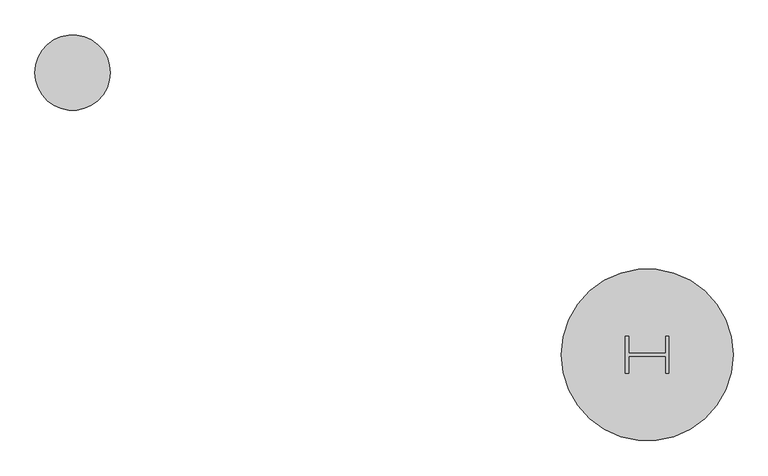
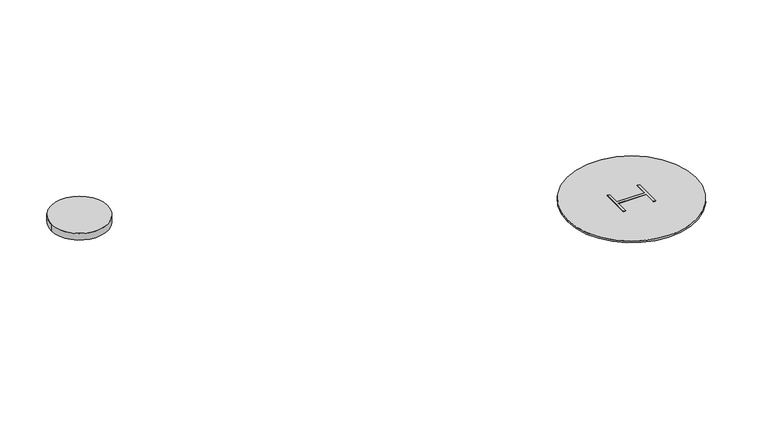
"""IFC4 building model written with IfcOpenShell, lengths in millimetres: proxy geometry."""

from ifc_helpers import new_model, si_unit, point, frame_2d, origin, origin_with_axes, place, context, project, spatial, polyline, circle_curve, trimmed, segment, composite_curve, outline, extrude, source, transform, mapped, element, save


def roads_7a27419f(model_context):
    return source(origin(), model_context, "Body", "SweptSolid", [
        extrude(outline(composite_curve([segment(trimmed(circle_curve(frame_2d((22641.7428665, -13142.2373856)), 2823.6884968), [point((19818.0543697, -13142.2373856))], [point((25465.4313633, -13142.2373856))], False, "CARTESIAN"), True, "CONTINUOUS"), segment(trimmed(circle_curve(frame_2d((22641.7428665, -13142.2373856)), 2823.6884968), [point((25465.4313633, -13142.2373856))], [point((19818.0543697, -13142.2373856))], False, "CARTESIAN"), True, "CONTINUOUS")], self_intersect=False)), origin_with_axes(), (0.0, 0.0, 1.0), 76.2),
        extrude(outline(polyline([(23352.9428665, -12532.6373856), (23352.9428665, -13751.8373856), (23251.3428665, -13751.8373856), (23251.3428665, -13193.0373856), (22032.1428665, -13193.0373856), (22032.1428665, -13751.8373856), (21930.5428665, -13751.8373856), (21930.5428665, -12532.6373856), (22032.1428665, -12532.6373856), (22032.1428665, -13091.4373856), (23251.3428665, -13091.4373856), (23251.3428665, -12532.6373856), (23352.9428665, -12532.6373856)])), origin_with_axes(), (0.0, 0.0, 1.0), 101.6),
        extrude(outline(composite_curve([segment(trimmed(circle_curve(frame_2d((3774.4468549, -3874.163359)), 1237.2277501), [point((2537.2191048, -3874.163359))], [point((5011.6746051, -3874.163359))], False, "CARTESIAN"), True, "CONTINUOUS"), segment(trimmed(circle_curve(frame_2d((3774.4468549, -3874.163359)), 1237.2277501), [point((5011.6746051, -3874.163359))], [point((2537.2191048, -3874.163359))], False, "CARTESIAN"), True, "CONTINUOUS")], self_intersect=False)), origin_with_axes(), (0.0, 0.0, 1.0), 304.8),
    ])


if __name__ == "__main__":
    model = new_model("IFC4")
    model_context = context("Model", 3, world=origin())
    ifc_project = project(units=[si_unit("LENGTHUNIT", "METRE", prefix="MILLI")], contexts=[model_context])
    site = spatial("IfcSite", under=ifc_project)
    building = spatial("IfcBuilding", under=site)
    placement = place(None, origin())
    roads_shape = roads_7a27419f(model_context)
    element("IfcBuildingElementProxy", 1, Name="Roads", at=placement, inside=building, context=model_context, shape_type="MappedRepresentation", body=[
        mapped(roads_shape, transform((0.0, 0.0, 0.0), x_axis=(1.0, 0.0, 0.0), y_axis=(0.0, 1.0, 0.0), z_axis=(0.0, 0.0, 1.0))),
    ])
    save(model, "model.ifc")

# Revit data of these elements
# Element 1 (IfcBuildingElementProxy)
#   Materials on its faces: "ROAD"
# Materials
#   "ROAD": class "Generic", colour RGB 120 120 120, transparency 0, Cost = 0
